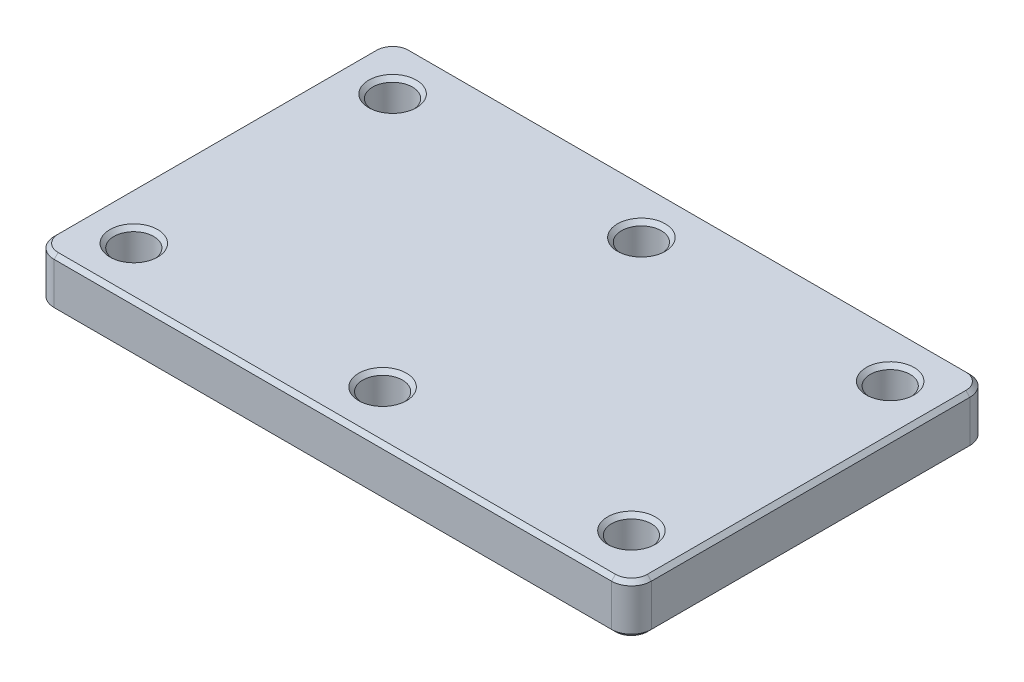
SolidWorks part; units mm, degrees
material "Plain Carbon Steel"
ref_plane "Front Plane" through (0, 0, 0) normal (0, 0, 1) x (1, 0, 0)
ref_plane "Top Plane" through (0, 0, 0) normal (0, 1, 0) x (1, 0, 0)
ref_plane "Right Plane" through (0, 0, 0) normal (1, 0, 0) x (0, 0, -1)
sketch "Plate Outline and Hole Sketch" plane through (0, 0, 0) normal (0, 1, 0) x (1, 0, 0)
  line L0 (-13.75, 0) -> (13.75, 0) construction
  line L1 (-140, 90) -> (140, 90)
  line L2 (-150, 80) -> (-150, -80)
  line L3 (-140, -90) -> (140, -90)
  line L4 (150, 80) -> (150, -80)
  line L5 (-150, 90) -> (150, -90) construction
  line L6 (-150, -90) -> (150, 90) construction
  line L7 (0, -13.75) -> (0, 13.75) construction
  arc A0 (140, 90) -> (150, 80) centre (140, 80) cw
  arc A1 (-140, 90) -> (-150, 80) centre (-140, 80) ccw
  arc A2 (140, -90) -> (150, -80) centre (140, -80) ccw
  arc A3 (-150, -80) -> (-140, -90) centre (-140, -80) ccw
  circle A4 centre (-125, 65) radius 10
  circle A5 centre (-125, -65) radius 10
  circle A6 centre (125, 65) radius 10
  circle A7 centre (125, -65) radius 10
  circle A8 centre (0, 65) radius 10
  circle A9 centre (0, -65) radius 10
  point P0 (0, 0)
  dimension "D3" = 10
  dimension "D4" = 20
  dimension "D7" = 20
  dimension "D1" = 300
  dimension "D2" = 180
  dimension "D5" = 250
  dimension "D6" = 130
extrude "Base Plate 25mm" add sketch "Plate Outline and Hole Sketch" along normal blind 25
chamfer "Edge Chamfer 2x45deg" distance 2 angle 45 28 edges at (125, 0, 75) (-125, 0, 55) (0, 0, -90) (-147.0711, 0, -87.0711) (-150, 0, 0) (-147.0711, 0, 87.0711) (0, 0, 90) (147.0711, 0, 87.0711) (150, 0, 0) (147.0711, 0, -87.0711) (-125, 0, -55) (125, 0, -75) (125, 25, 75) (125, 25, -75) (-125, 25, 55) (-125, 25, -55) (150, 25, 0) (147.0711, 25, 87.0711) (0, 25, 90) (-147.0711, 25, 87.0711) (-150, 25, 0) (-147.0711, 25, -87.0711) (0, 25, -90) (147.0711, 25, -87.0711) (0, 0, 75) (0, 0, -55) (0, 25, 75) (0, 25, -55)
